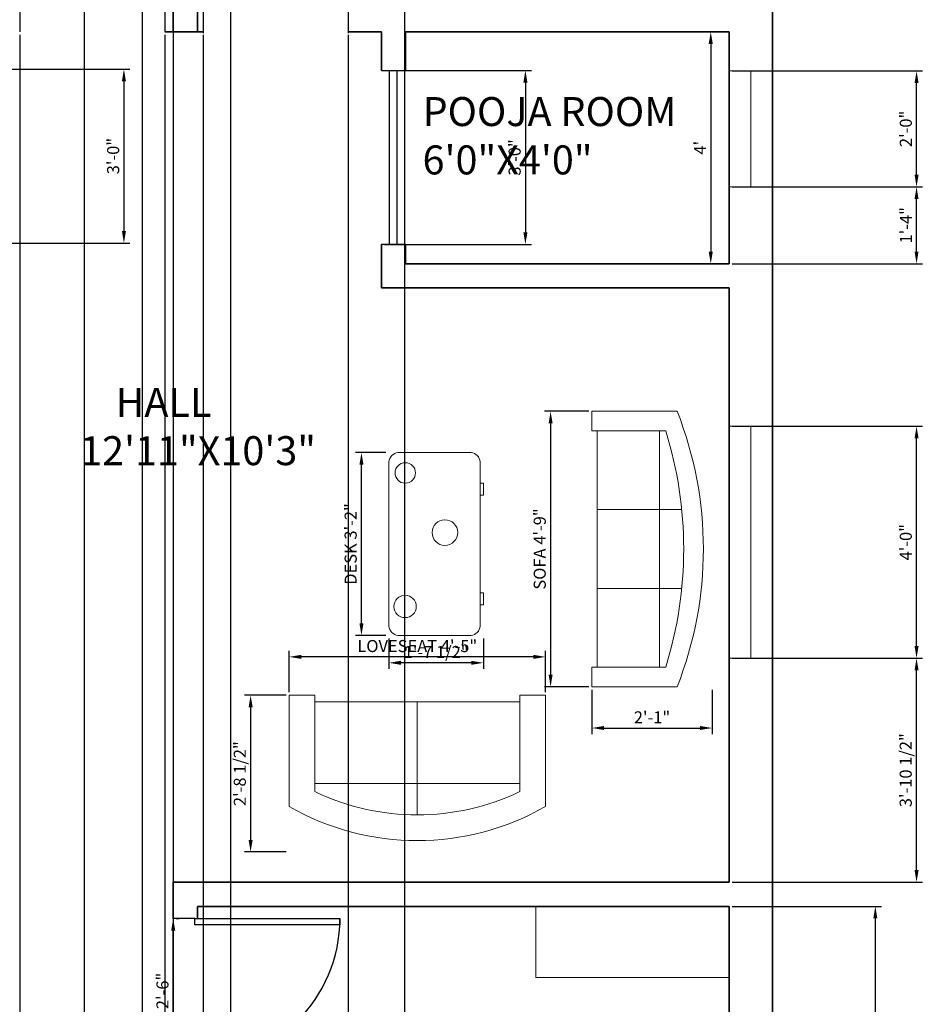
# Model space of a CAD drawing. Units: inches. Extents: x 3889 to 4254, y 3310 to 3958.
# Tile 4 of 6: x 4067 to 4254, y 3534 to 3738. Entities that reach past the tile are written whole.
import ezdxf

# ---------------------------------------------------------------- set-up
doc = ezdxf.new("R2010")
doc.units = ezdxf.units.IN
for name, color, linetype, lineweight in [('A-AREA-IDEN', 11, 'Continuous', 18), ('A-WALL', 7, 'Continuous', 35), ('DIM', 81, 'Continuous', 18), ('DOOR', 1, 'Continuous', 25), ('FURNITURES', 130, 'Continuous', 18), ('WINDOW', 3, 'Continuous', 18)]:
    doc.layers.add(name, color=color, linetype=linetype, lineweight=lineweight)
doc.styles.get("Standard").update_dxf_attribs({"font": 'arial.ttf'})
doc.dimstyles.new('ISO-25', dxfattribs={"dimtxt": 2.5, "dimasz": 2.5, "dimexe": 1.25, "dimexo": 0.625, "dimtad": 1, "dimlunit": 3, "dimtxsty": 'Standard', "dimcen": 2.5, "dimadec": 0, "dimazin": 0, "dimtfac": 1, "dimtmove": 0, "dimatfit": 3, "dimfxl": 1, "dimarcsym": 0})

# ---------------------------------------------------------------- blocks, each defined once
blk = doc.blocks.new('*U4')
for p, q in [((0, 0), (0, -6)), ((40, 0), (40, -6))]:
    blk.add_line(p, q)
blk.add_lwpolyline([(0, 0), (0, 40), (1.75, 40), (1.75, 0)], close=True)
blk.add_arc((0, 0), 40, 0, 90)
blk = doc.blocks.new('*U2')
for p, q in [((0, 0), (0, -6)), ((-40, 0), (-40, -6))]:
    blk.add_line(p, q)
blk.add_lwpolyline([(0, 0), (0, 40), (-1.75, 40), (-1.75, 0)], close=True)
blk.add_arc((0, 0), 40, 90, 180)
blk = doc.blocks.new('*U3')
for p, q in [((-40, 0), (-40, 6)), ((0, 0), (0, 6))]:
    blk.add_line(p, q)
blk.add_lwpolyline([(0, 0), (0, -40), (-1.75, -40), (-1.75, 0)], close=True)
blk.add_arc((0, 0), 40, 180, 270)
blk = doc.blocks.new('Desk - 30 x 60 in.')
for p, q in [((-26.999995, 0), (26.999995, 0)), ((-29.999995, -27), (-29.999995, -3)), ((29.999995, -3), (29.999995, -27)), ((26.999995, -30), (-26.999995, -30)), ((-20.000005, -30), (-20.000005, -31)), ((-20.000005, -31), (-16.000005, -31)), ((-16.000005, -31), (-16.000005, -30)), ((15.999995, -31), (15.999995, -30)), ((19.999995, -31), (15.999995, -31)), ((19.999995, -30), (19.999995, -31))]:
    blk.add_line(p, q)
for centre, start, end in [((-26.499995, -3.5), 98.1301, 171.8699), ((26.499995, -3.5), 8.130102, 81.8699), ((-26.499995, -26.5), 188.1301, 261.8699), ((26.499995, -26.5), 278.1301, 351.8699)]:
    blk.add_arc(centre, 3.535534, start, end)
blk = doc.blocks.new('Sofa - Roundback 7 ft.')
for p, q in [((-12.00002, -32.4421), (-12.00003, -6.5971)), ((11.99997, -32.4421), (11.99998, -6.5971)), ((-36.000027, -34), (-36.000027, -11.4696)), ((35.99998, -34), (35.99998, -11.4696)), ((-35.999844, -13.3819), (35.9998, -13.3819)), ((-36.000027, -32.4421), (35.99998, -32.4421))]:
    blk.add_line(p, q)
for points in [[(-36.000027, -34), (-42.000027, -34), (-42.000027, -8)], [(41.99998, -8), (41.99998, -34), (35.99998, -34)]]:
    blk.add_lwpolyline(points)
for centre, radius, start, end in [((0, -114.25), 114.25, 68.43141, 111.5686), ((-0.00001, -127.1968), 121.1968, 72.72033, 107.2797)]:
    blk.add_arc(centre, radius, start, end)
blk = doc.blocks.new('Sofa - Roundback Loveseat 5 ft.')
for p, q in [((0, -32.44198), (0, -5.99998)), ((-24, -33.99998), (-24, -11.46958)), ((24.00004, -33.99998), (24.00004, -11.46958)), ((-23.9998, -13.38178), (23.99986, -13.38178)), ((-24, -32.44198), (24.00004, -32.44198))]:
    blk.add_line(p, q)
for points in [[(-24, -33.99998), (-30, -33.99998), (-30, -7.99998)], [(30.00004, -7.99998), (30.00004, -33.99998), (24.00004, -33.99998)]]:
    blk.add_lwpolyline(points)
for centre, radius, start, end in [((0, -60.24998), 60.24998, 60.13715, 119.8628), ((0, -61.38438), 55.38444, 64.32083, 115.6792)]:
    blk.add_arc(centre, radius, start, end)
blk = doc.blocks.new('*D27')
at = {"layer": 'Defpoints', "color": 0, "transparency": 16777216}
for p in [(4098.84, 3551.61), (4098.84, 3551.61), (4098.84, 3521.61)]:
    blk.add_point(p, dxfattribs=at)
at = {"layer": 'DIM', "color": 0, "lineweight": -2, "transparency": 16777216}
for p, q in [((4099.47, 3551.61), (4100.09, 3551.61)), ((4098.84, 3524.11), (4098.84, 3549.11)), ((4099.47, 3521.61), (4100.09, 3521.61))]:
    blk.add_line(p, q, dxfattribs=at)
at = {"layer": 'DIM', "color": 0, "transparency": 16777216}
for points in [[(4098.43, 3549.11), (4099.26, 3549.11), (4098.84, 3551.61)], [(4098.43, 3524.11), (4099.26, 3524.11), (4098.84, 3521.61)]]:
    blk.add_solid(points, dxfattribs=at)
at = {"layer": 'DIM', "color": 0, "transparency": 16777216, "insert": (4096.94, 3536.61), "char_height": 2.5, "attachment_point": 5, "rotation": 90}
blk.add_mtext('2\'-6"', dxfattribs=at)
blk = doc.blocks.new('*D29')
at = {"layer": 'Defpoints', "color": 0, "transparency": 16777216}
for p in [(4213.84, 3554.11), (4213.84, 3434.11), (4244.11, 3434.11)]:
    blk.add_point(p, dxfattribs=at)
at = {"layer": 'DIM', "color": 0, "lineweight": -2, "transparency": 16777216}
for p, q in [((4214.47, 3554.11), (4245.36, 3554.11)), ((4244.11, 3551.61), (4244.11, 3436.61)), ((4214.47, 3434.11), (4245.36, 3434.11))]:
    blk.add_line(p, q, dxfattribs=at)
at = {"layer": 'DIM', "color": 0, "transparency": 16777216}
for points in [[(4243.7, 3551.61), (4244.53, 3551.61), (4244.11, 3554.11)], [(4243.7, 3436.61), (4244.53, 3436.61), (4244.11, 3434.11)]]:
    blk.add_solid(points, dxfattribs=at)
at = {"layer": 'DIM', "color": 0, "transparency": 16777216, "insert": (4242.21, 3494.11), "char_height": 2.5, "attachment_point": 5, "rotation": 90}
blk.add_mtext("10'", dxfattribs=at)
blk = doc.blocks.new('*D30')
at = {"layer": 'Defpoints', "color": 0, "transparency": 16777216}
for p in [(4208.35, 3735.11), (4208.35, 3687.11), (4210.06, 3687.11)]:
    blk.add_point(p, dxfattribs=at)
at = {"layer": 'DIM', "color": 0, "lineweight": -2, "transparency": 16777216}
for p, q in [((4208.98, 3735.11), (4211.31, 3735.11)), ((4210.06, 3732.61), (4210.06, 3689.61)), ((4208.98, 3687.11), (4211.31, 3687.11))]:
    blk.add_line(p, q, dxfattribs=at)
at = {"layer": 'DIM', "color": 0, "transparency": 16777216}
for points in [[(4209.64, 3732.61), (4210.48, 3732.61), (4210.06, 3735.11)], [(4209.64, 3689.61), (4210.48, 3689.61), (4210.06, 3687.11)]]:
    blk.add_solid(points, dxfattribs=at)
at = {"layer": 'DIM', "color": 0, "transparency": 16777216, "insert": (4208.18, 3711.11), "char_height": 2.5, "attachment_point": 5, "rotation": 90}
blk.add_mtext("4'", dxfattribs=at)
blk = doc.blocks.new('WIN-48x9')
blk.add_line((4.5, 48), (4.5, 0))
blk.add_lwpolyline([(0, 48), (9, 48), (9, 0), (0, 0)], close=True)
blk = doc.blocks.new('WIN-24x9')
blk.add_line((24, 4.5), (0, 4.5))
blk.add_lwpolyline([(24, 9), (24, 0), (0, 0), (0, 9)], close=True)
blk = doc.blocks.new('*D53')
at = {"layer": 'Defpoints', "color": 0, "transparency": 16777216}
for p in [(4137.79, 3648.02), (4143.47, 3648.02), (4143.47, 3610.19)]:
    blk.add_point(p, dxfattribs=at)
at = {"layer": 'DIM', "color": 0, "lineweight": -2, "transparency": 16777216}
for p, q in [((4142.84, 3648.02), (4136.54, 3648.02)), ((4137.79, 3612.69), (4137.79, 3645.52)), ((4142.84, 3610.19), (4136.54, 3610.19))]:
    blk.add_line(p, q, dxfattribs=at)
at = {"layer": 'DIM', "color": 0, "transparency": 16777216}
for points in [[(4137.38, 3645.52), (4138.21, 3645.52), (4137.79, 3648.02)], [(4137.38, 3612.69), (4138.21, 3612.69), (4137.79, 3610.19)]]:
    blk.add_solid(points, dxfattribs=at)
at = {"layer": 'DIM', "color": 0, "transparency": 16777216, "insert": (4135.88, 3629.1), "char_height": 2.5, "attachment_point": 5, "rotation": 90}
blk.add_mtext('DESK 3\'-2"', dxfattribs=at)
blk = doc.blocks.new('*D54')
at = {"layer": 'Defpoints', "color": 0, "transparency": 16777216}
for p in [(4143.47, 3610.19), (4163.01, 3610.19), (4143.47, 3604.51)]:
    blk.add_point(p, dxfattribs=at)
at = {"layer": 'DIM', "color": 0, "lineweight": -2, "transparency": 16777216}
for p, q in [((4143.47, 3609.56), (4143.47, 3603.26)), ((4163.01, 3609.56), (4163.01, 3603.26)), ((4160.51, 3604.51), (4145.97, 3604.51))]:
    blk.add_line(p, q, dxfattribs=at)
at = {"layer": 'DIM', "color": 0, "transparency": 16777216}
for points in [[(4145.97, 3604.93), (4145.97, 3604.1), (4143.47, 3604.51)], [(4160.51, 3604.93), (4160.51, 3604.1), (4163.01, 3604.51)]]:
    blk.add_solid(points, dxfattribs=at)
at = {"layer": 'DIM', "color": 0, "transparency": 16777216, "insert": (4153.24, 3606.43), "char_height": 2.5, "attachment_point": 5}
blk.add_mtext('1\'-7 1/2"', dxfattribs=at)
blk = doc.blocks.new('*D55')
at = {"layer": 'Defpoints', "color": 0, "transparency": 16777216}
for p in [(4185.47, 3656.56), (4176.92, 3599.57), (4185.47, 3599.57)]:
    blk.add_point(p, dxfattribs=at)
at = {"layer": 'DIM', "color": 0, "lineweight": -2, "transparency": 16777216}
for p, q in [((4184.85, 3656.56), (4175.67, 3656.56)), ((4176.92, 3654.06), (4176.92, 3602.07)), ((4184.85, 3599.57), (4175.67, 3599.57))]:
    blk.add_line(p, q, dxfattribs=at)
at = {"layer": 'DIM', "color": 0, "transparency": 16777216}
for points in [[(4176.51, 3654.06), (4177.34, 3654.06), (4176.92, 3656.56)], [(4176.51, 3602.07), (4177.34, 3602.07), (4176.92, 3599.57)]]:
    blk.add_solid(points, dxfattribs=at)
at = {"layer": 'DIM', "color": 0, "transparency": 16777216, "insert": (4175, 3628.07), "char_height": 2.5, "attachment_point": 5, "rotation": 90}
blk.add_mtext('SOFA 4\'-9"', dxfattribs=at)
blk = doc.blocks.new('*D56')
at = {"layer": 'Defpoints', "color": 0, "transparency": 16777216}
for p in [(4185.47, 3599.57), (4210.35, 3599.57), (4210.35, 3591.02)]:
    blk.add_point(p, dxfattribs=at)
at = {"layer": 'DIM', "color": 0, "lineweight": -2, "transparency": 16777216}
for p, q in [((4185.47, 3598.95), (4185.47, 3589.77)), ((4210.35, 3598.95), (4210.35, 3589.77)), ((4187.97, 3591.02), (4207.85, 3591.02))]:
    blk.add_line(p, q, dxfattribs=at)
at = {"layer": 'DIM', "color": 0, "transparency": 16777216}
for points in [[(4187.97, 3591.44), (4187.97, 3590.61), (4185.47, 3591.02)], [(4207.85, 3591.44), (4207.85, 3590.61), (4210.35, 3591.02)]]:
    blk.add_solid(points, dxfattribs=at)
at = {"layer": 'DIM', "color": 0, "transparency": 16777216, "insert": (4197.91, 3592.9), "char_height": 2.5, "attachment_point": 5}
blk.add_mtext('2\'-1"', dxfattribs=at)
blk = doc.blocks.new('*D57')
at = {"layer": 'Defpoints', "color": 0, "transparency": 16777216}
for p in [(4122.82, 3605.74), (4122.82, 3597.79), (4175.87, 3597.79)]:
    blk.add_point(p, dxfattribs=at)
at = {"layer": 'DIM', "color": 0, "lineweight": -2, "transparency": 16777216}
for p, q in [((4122.82, 3598.41), (4122.82, 3606.99)), ((4175.87, 3598.41), (4175.87, 3606.99)), ((4173.37, 3605.74), (4125.32, 3605.74))]:
    blk.add_line(p, q, dxfattribs=at)
at = {"layer": 'DIM', "color": 0, "transparency": 16777216}
for points in [[(4125.32, 3606.16), (4125.32, 3605.33), (4122.82, 3605.74)], [(4173.37, 3606.16), (4173.37, 3605.33), (4175.87, 3605.74)]]:
    blk.add_solid(points, dxfattribs=at)
at = {"layer": 'DIM', "color": 0, "transparency": 16777216, "insert": (4149.34, 3607.66), "char_height": 2.5, "attachment_point": 5}
blk.add_mtext('LOVESEAT 4\'-5"', dxfattribs=at)
blk = doc.blocks.new('*D58')
at = {"layer": 'Defpoints', "color": 0, "transparency": 16777216}
for p in [(4122.82, 3597.79), (4114.86, 3565.37), (4122.82, 3565.37)]:
    blk.add_point(p, dxfattribs=at)
at = {"layer": 'DIM', "color": 0, "lineweight": -2, "transparency": 16777216}
for p, q in [((4122.19, 3597.79), (4113.61, 3597.79)), ((4114.86, 3595.29), (4114.86, 3567.87)), ((4122.19, 3565.37), (4113.61, 3565.37))]:
    blk.add_line(p, q, dxfattribs=at)
at = {"layer": 'DIM', "color": 0, "transparency": 16777216}
for points in [[(4114.44, 3595.29), (4115.28, 3595.29), (4114.86, 3597.79)], [(4114.44, 3567.87), (4115.28, 3567.87), (4114.86, 3565.37)]]:
    blk.add_solid(points, dxfattribs=at)
at = {"layer": 'DIM', "color": 0, "transparency": 16777216, "insert": (4112.94, 3581.58), "char_height": 2.5, "attachment_point": 5, "rotation": 90}
blk.add_mtext('2\'-8 1/2"', dxfattribs=at)
blk = doc.blocks.new('*D71')
at = {"layer": 'Defpoints', "color": 0, "transparency": 16777216}
for p in [(4092.52, 3951.91), (4080.52, 3351.11), (4092.52, 3351.11)]:
    blk.add_point(p, dxfattribs=at)
at = {"layer": 'DIM', "color": 0, "lineweight": -2, "transparency": 16777216}
for p, q in [((4080.52, 3351.73), (4080.52, 3953.16)), ((4092.52, 3351.73), (4092.52, 3953.16)), ((4083.02, 3951.91), (4090.02, 3951.91))]:
    blk.add_line(p, q, dxfattribs=at)
at = {"layer": 'DIM', "color": 0, "transparency": 16777216}
for points in [[(4083.02, 3952.32), (4083.02, 3951.49), (4080.52, 3951.91)], [(4090.02, 3952.32), (4090.02, 3951.49), (4092.52, 3951.91)]]:
    blk.add_solid(points, dxfattribs=at)
at = {"layer": 'DIM', "color": 0, "transparency": 16777216, "insert": (4086.52, 3953.81), "char_height": 2.5, "attachment_point": 5}
blk.add_mtext('1\'-0"', dxfattribs=at)
blk = doc.blocks.new('*D78')
at = {"layer": 'Defpoints', "color": 0, "transparency": 16777216}
for p in [(4213.84, 3703.01), (4252.64, 3703.01), (4213.84, 3687.11)]:
    blk.add_point(p, dxfattribs=at)
at = {"layer": 'DIM', "color": 0, "lineweight": -2, "transparency": 16777216}
for p, q in [((4214.47, 3703.01), (4253.89, 3703.01)), ((4252.64, 3689.61), (4252.64, 3700.51)), ((4214.47, 3687.11), (4253.89, 3687.11))]:
    blk.add_line(p, q, dxfattribs=at)
at = {"layer": 'DIM', "color": 0, "transparency": 16777216}
for points in [[(4252.23, 3700.51), (4253.06, 3700.51), (4252.64, 3703.01)], [(4252.23, 3689.61), (4253.06, 3689.61), (4252.64, 3687.11)]]:
    blk.add_solid(points, dxfattribs=at)
at = {"layer": 'DIM', "color": 0, "transparency": 16777216, "insert": (4250.76, 3695.06), "char_height": 2.5, "attachment_point": 5, "rotation": 90}
blk.add_mtext('1\'-4"', dxfattribs=at)
blk = doc.blocks.new('*D79')
at = {"layer": 'Defpoints', "color": 0, "transparency": 16777216}
for p in [(4213.84, 3605.47), (4252.64, 3605.47), (4213.84, 3559.11)]:
    blk.add_point(p, dxfattribs=at)
at = {"layer": 'DIM', "color": 0, "lineweight": -2, "transparency": 16777216}
for p, q in [((4214.47, 3605.47), (4253.89, 3605.47)), ((4252.64, 3561.61), (4252.64, 3602.97)), ((4214.47, 3559.11), (4253.89, 3559.11))]:
    blk.add_line(p, q, dxfattribs=at)
at = {"layer": 'DIM', "color": 0, "transparency": 16777216}
for points in [[(4252.23, 3602.97), (4253.06, 3602.97), (4252.64, 3605.47)], [(4252.23, 3561.61), (4253.06, 3561.61), (4252.64, 3559.11)]]:
    blk.add_solid(points, dxfattribs=at)
at = {"layer": 'DIM', "color": 0, "transparency": 16777216, "insert": (4250.72, 3582.29), "char_height": 2.5, "attachment_point": 5, "rotation": 90}
blk.add_mtext('3\'-10 1/2"', dxfattribs=at)
blk = doc.blocks.new('*D83')
at = {"layer": 'Defpoints', "color": 0, "transparency": 16777216}
for p in [(4213.84, 3653.47), (4252.64, 3653.47), (4213.84, 3605.47)]:
    blk.add_point(p, dxfattribs=at)
at = {"layer": 'DIM', "color": 0, "lineweight": -2, "transparency": 16777216}
for p, q in [((4214.47, 3653.47), (4253.89, 3653.47)), ((4252.64, 3607.97), (4252.64, 3650.97)), ((4214.47, 3605.47), (4253.89, 3605.47))]:
    blk.add_line(p, q, dxfattribs=at)
at = {"layer": 'DIM', "color": 0, "transparency": 16777216}
for points in [[(4252.23, 3650.97), (4253.06, 3650.97), (4252.64, 3653.47)], [(4252.23, 3607.97), (4253.06, 3607.97), (4252.64, 3605.47)]]:
    blk.add_solid(points, dxfattribs=at)
at = {"layer": 'DIM', "color": 0, "transparency": 16777216, "insert": (4250.74, 3629.47), "char_height": 2.5, "attachment_point": 5, "rotation": 90}
blk.add_mtext('4\'-0"', dxfattribs=at)
blk = doc.blocks.new('*D84')
at = {"layer": 'Defpoints', "color": 0, "transparency": 16777216}
for p in [(4213.84, 3727.01), (4252.64, 3727.01), (4213.84, 3703.01)]:
    blk.add_point(p, dxfattribs=at)
at = {"layer": 'DIM', "color": 0, "lineweight": -2, "transparency": 16777216}
for p, q in [((4214.47, 3727.01), (4253.89, 3727.01)), ((4252.64, 3705.51), (4252.64, 3724.51)), ((4214.47, 3703.01), (4253.89, 3703.01))]:
    blk.add_line(p, q, dxfattribs=at)
at = {"layer": 'DIM', "color": 0, "transparency": 16777216}
for points in [[(4252.23, 3724.51), (4253.06, 3724.51), (4252.64, 3727.01)], [(4252.23, 3705.51), (4253.06, 3705.51), (4252.64, 3703.01)]]:
    blk.add_solid(points, dxfattribs=at)
at = {"layer": 'DIM', "color": 0, "transparency": 16777216, "insert": (4250.74, 3715.01), "char_height": 2.5, "attachment_point": 5, "rotation": 90}
blk.add_mtext('2\'-0"', dxfattribs=at)
blk = doc.blocks.new('*D85')
at = {"layer": 'Defpoints', "color": 0, "transparency": 16777216}
for p in [(4110.69, 3860.11), (4146.69, 3860.11), (4146.69, 3312.31)]:
    blk.add_point(p, dxfattribs=at)
at = {"layer": 'DIM', "color": 0, "lineweight": -2, "transparency": 16777216}
for p, q in [((4110.69, 3859.48), (4110.69, 3311.06)), ((4146.69, 3859.48), (4146.69, 3311.06)), ((4113.19, 3312.31), (4144.19, 3312.31))]:
    blk.add_line(p, q, dxfattribs=at)
at = {"layer": 'DIM', "color": 0, "transparency": 16777216}
for points in [[(4113.19, 3312.72), (4113.19, 3311.89), (4110.69, 3312.31)], [(4144.19, 3312.72), (4144.19, 3311.89), (4146.69, 3312.31)]]:
    blk.add_solid(points, dxfattribs=at)
at = {"layer": 'DIM', "color": 0, "transparency": 16777216, "insert": (4128.69, 3314.21), "char_height": 2.5, "attachment_point": 5}
blk.add_mtext('3\'-0"', dxfattribs=at)
blk = doc.blocks.new('*D86')
at = {"layer": 'Defpoints', "color": 0, "transparency": 16777216}
for p in [(4046.84, 3865.11), (4110.69, 3865.11), (4110.69, 3312.31)]:
    blk.add_point(p, dxfattribs=at)
at = {"layer": 'DIM', "color": 0, "lineweight": -2, "transparency": 16777216}
for p, q in [((4046.84, 3864.48), (4046.84, 3311.06)), ((4110.69, 3864.48), (4110.69, 3311.06)), ((4049.34, 3312.31), (4108.19, 3312.31))]:
    blk.add_line(p, q, dxfattribs=at)
at = {"layer": 'DIM', "color": 0, "transparency": 16777216}
for points in [[(4049.34, 3312.72), (4049.34, 3311.89), (4046.84, 3312.31)], [(4108.19, 3312.72), (4108.19, 3311.89), (4110.69, 3312.31)]]:
    blk.add_solid(points, dxfattribs=at)
at = {"layer": 'DIM', "color": 0, "transparency": 16777216, "insert": (4078.77, 3314.2), "char_height": 2.5, "attachment_point": 5}
blk.add_mtext('5\'-4"', dxfattribs=at)
blk = doc.blocks.new('*D87')
at = {"layer": 'Defpoints', "color": 0, "transparency": 16777216}
for p in [(4058.84, 3727.38), (4058.84, 3691.38), (4088.64, 3691.38)]:
    blk.add_point(p, dxfattribs=at)
at = {"layer": 'DIM', "color": 0, "lineweight": -2, "transparency": 16777216}
for p, q in [((4059.47, 3727.38), (4089.89, 3727.38)), ((4088.64, 3724.88), (4088.64, 3693.88)), ((4059.47, 3691.38), (4089.89, 3691.38))]:
    blk.add_line(p, q, dxfattribs=at)
at = {"layer": 'DIM', "color": 0, "transparency": 16777216}
for points in [[(4088.23, 3724.88), (4089.06, 3724.88), (4088.64, 3727.38)], [(4088.23, 3693.88), (4089.06, 3693.88), (4088.64, 3691.38)]]:
    blk.add_solid(points, dxfattribs=at)
at = {"layer": 'DIM', "color": 0, "transparency": 16777216, "insert": (4086.74, 3709.38), "char_height": 2.5, "attachment_point": 5, "rotation": 90}
blk.add_mtext('3\'-0"', dxfattribs=at)
blk = doc.blocks.new('*D88')
at = {"layer": 'Defpoints', "color": 0, "transparency": 16777216}
for p in [(4141.91, 3727.1), (4141.91, 3691.1), (4171.71, 3691.1)]:
    blk.add_point(p, dxfattribs=at)
at = {"layer": 'DIM', "color": 0, "lineweight": -2, "transparency": 16777216}
for p, q in [((4142.53, 3727.1), (4172.96, 3727.1)), ((4171.71, 3724.6), (4171.71, 3693.6)), ((4142.53, 3691.1), (4172.96, 3691.1))]:
    blk.add_line(p, q, dxfattribs=at)
at = {"layer": 'DIM', "color": 0, "transparency": 16777216}
for points in [[(4171.29, 3724.6), (4172.13, 3724.6), (4171.71, 3727.1)], [(4171.29, 3693.6), (4172.13, 3693.6), (4171.71, 3691.1)]]:
    blk.add_solid(points, dxfattribs=at)
at = {"layer": 'DIM', "color": 0, "transparency": 16777216, "insert": (4169.81, 3709.1), "char_height": 2.5, "attachment_point": 5, "rotation": 90}
blk.add_mtext('3\'-0"', dxfattribs=at)
blk = doc.blocks.new('*D89')
at = {"layer": 'Defpoints', "color": 0, "transparency": 16777216}
for p in [(4067.08, 3735.11), (4097.08, 3735.11), (4097.08, 3312.31)]:
    blk.add_point(p, dxfattribs=at)
at = {"layer": 'DIM', "color": 0, "lineweight": -2, "transparency": 16777216}
for p, q in [((4067.08, 3734.48), (4067.08, 3311.06)), ((4097.08, 3734.48), (4097.08, 3311.06)), ((4069.58, 3312.31), (4094.58, 3312.31))]:
    blk.add_line(p, q, dxfattribs=at)
at = {"layer": 'DIM', "color": 0, "transparency": 16777216}
for points in [[(4069.58, 3312.72), (4069.58, 3311.89), (4067.08, 3312.31)], [(4094.58, 3312.72), (4094.58, 3311.89), (4097.08, 3312.31)]]:
    blk.add_solid(points, dxfattribs=at)
at = {"layer": 'DIM', "color": 0, "transparency": 16777216, "insert": (4082.08, 3314.21), "char_height": 2.5, "attachment_point": 5}
blk.add_mtext('2\'-6"', dxfattribs=at)
blk = doc.blocks.new('*D90')
at = {"layer": 'Defpoints', "color": 0, "transparency": 16777216}
for p in [(4105.04, 3735.11), (4135.04, 3735.11), (4135.04, 3312.31)]:
    blk.add_point(p, dxfattribs=at)
at = {"layer": 'DIM', "color": 0, "lineweight": -2, "transparency": 16777216}
for p, q in [((4105.04, 3734.48), (4105.04, 3311.06)), ((4135.04, 3734.48), (4135.04, 3311.06)), ((4107.54, 3312.31), (4132.54, 3312.31))]:
    blk.add_line(p, q, dxfattribs=at)
at = {"layer": 'DIM', "color": 0, "transparency": 16777216}
for points in [[(4107.54, 3312.72), (4107.54, 3311.89), (4105.04, 3312.31)], [(4132.54, 3312.72), (4132.54, 3311.89), (4135.04, 3312.31)]]:
    blk.add_solid(points, dxfattribs=at)
at = {"layer": 'DIM', "color": 0, "transparency": 16777216, "insert": (4120.04, 3314.21), "char_height": 2.5, "attachment_point": 5}
blk.add_mtext('2\'-6"', dxfattribs=at)
blk = doc.blocks.new('*D95')
at = {"layer": 'Defpoints', "color": 0, "transparency": 16777216}
for p in [(4046.84, 3865.11), (4098.84, 3860.11), (4098.84, 3312.31)]:
    blk.add_point(p, dxfattribs=at)
at = {"layer": 'DIM', "color": 0, "lineweight": -2, "transparency": 16777216}
for p, q in [((4046.84, 3864.48), (4046.84, 3311.06)), ((4098.84, 3859.48), (4098.84, 3311.06)), ((4049.34, 3312.31), (4096.34, 3312.31))]:
    blk.add_line(p, q, dxfattribs=at)
at = {"layer": 'DIM', "color": 0, "transparency": 16777216}
for points in [[(4049.34, 3312.72), (4049.34, 3311.89), (4046.84, 3312.31)], [(4096.34, 3312.72), (4096.34, 3311.89), (4098.84, 3312.31)]]:
    blk.add_solid(points, dxfattribs=at)
at = {"layer": 'DIM', "color": 0, "transparency": 16777216, "insert": (4072.84, 3314.18), "char_height": 2.5, "attachment_point": 5}
blk.add_mtext('4\'-4"', dxfattribs=at)

msp = doc.modelspace()

# ---------------------------------------------------------------- linework, layer by layer
at = {"layer": 'A-WALL'}
for p, q in [((4222.843, 3342.107), (4222.843, 3922.107)), ((4098.843, 3735.107), (4098.843, 3860.107)), ((4103.843, 3735.107), (4103.843, 3860.107)), ((4097.08, 3735.107), (4103.843, 3735.107)), ((4098.843, 3735.107), (4103.843, 3735.107)), ((4103.843, 3735.107), (4105.044, 3735.107)), ((4135.044, 3735.107), (4141.91, 3735.107)), ((4141.91, 3727.102), (4141.91, 3735.107)), ((4146.91, 3727.102), (4146.91, 3735.107)), ((4146.91, 3735.107), (4213.843, 3735.107)), ((4213.843, 3687.107), (4213.843, 3735.107)), ((4141.91, 3682.107), (4141.91, 3691.102)), ((4146.91, 3687.107), (4146.91, 3691.102)), ((4146.91, 3687.107), (4213.843, 3687.107)), ((4141.91, 3682.107), (4213.843, 3682.107)), ((4213.843, 3559.107), (4213.843, 3682.107)), ((4098.843, 3559.107), (4213.843, 3559.107)), ((4098.843, 3551.612), (4098.843, 3559.107)), ((4103.843, 3554.107), (4213.843, 3554.107)), ((4103.843, 3551.612), (4103.843, 3554.107)), ((4213.843, 3434.107), (4213.843, 3554.107))]:
    msp.add_line(p, q, dxfattribs=at)
at = {"layer": 'DOOR'}
for points in [[(4141.91, 3727.102), (4146.91, 3727.102)], [(4146.91, 3691.102), (4141.91, 3691.102)]]:
    msp.add_lwpolyline(points, dxfattribs=at)
msp.add_lwpolyline([(4143.572, 3727.102), (4145.076, 3727.102), (4145.076, 3691.102), (4143.572, 3691.102)], close=True, dxfattribs=at)
at = {"layer": 'FURNITURES'}
msp.add_lwpolyline([(4213.843, 3554.107), (4173.893, 3554.107), (4173.893, 3539.394), (4213.843, 3539.394)], close=True, dxfattribs=at)
for centre, radius in [((4146.861, 3643.814), 2.119), ((4155.058, 3631.466), 2.655), ((4146.809, 3616.181), 2.318)]:
    msp.add_circle(centre, radius, dxfattribs=at)

# ---------------------------------------------------------------- block references
at = {"layer": 'DOOR', "xscale": 0.75, "yscale": 0.75, "zscale": 0.75}
for name, p in [('*U2', (4097.08, 3739.607)), ('*U4', (4105.044, 3739.339))]:
    msp.add_blockref(name, p, dxfattribs=at)
at = {"layer": 'DOOR', "xscale": 0.75, "yscale": 0.75, "zscale": 0.75, "rotation": 90}
msp.add_blockref('*U3', (4103.343, 3551.612), dxfattribs=at)
at = {"layer": 'FURNITURES'}
for name, p, xscale, yscale, zscale, rotation in [('Sofa - Roundback 7 ft.', (4208.538, 3628.068), 0.6784518660872728, 0.6784518660872728, 0.6784518660872728, 270), ('Desk - 30 x 60 in.', (4143.468, 3629.103), 0.6305181038195912, 0.6305181038195912, 0.6305181038195912, 90), ('Sofa - Roundback Loveseat 5 ft.', (4149.343, 3567.724), 0.8841712959600512, 0.8841712959600512, 0.8841712959600512, 180)]:
    msp.add_blockref(name, p, dxfattribs=dict(at, xscale=xscale, yscale=yscale, zscale=zscale, rotation=rotation))
at = {"layer": 'WINDOW', "rotation": 89.99999999999939}
msp.add_blockref('WIN-24x9', (4222.843, 3703.007), dxfattribs=at)
at = {"layer": 'WINDOW'}
msp.add_blockref('WIN-48x9', (4213.843, 3605.469), dxfattribs=at)

# ---------------------------------------------------------------- texts
at = {"layer": 'A-AREA-IDEN', "char_height": 6, "attachment_point": 1}
for s, insert in [('POOJA ROOM\\P6\'0"X4\'0"', (4150.436, 3721.593)), ('    HALL\\P12\'11"X10\'3"', (4079.585, 3661.416))]:
    msp.add_mtext_dynamic_manual_height_columns(s, width=76.4548, gutter_width=12.5, heights=[0], dxfattribs=dict(at, insert=insert))

# ---------------------------------------------------------------- dimensions: what is measured, and where the dimension line sits
at = {"layer": 'DIM'}
for base, p1, p2, picture, middle in [((4092.518, 3951.907), (4080.518, 3351.107), (4092.518, 3351.107), '*D71', (4086.518, 3953.808)), ((4110.69, 3312.307), (4046.843, 3865.107), (4110.69, 3865.107), '*D86', (4078.766, 3314.203)), ((4098.843, 3312.307), (4046.843, 3865.107), (4098.843, 3860.107), '*D95', (4072.843, 3314.182)), ((4146.69, 3312.307), (4110.69, 3860.107), (4146.69, 3860.107), '*D85', (4128.69, 3314.209)), ((4097.08, 3312.307), (4067.08, 3735.107), (4097.08, 3735.107), '*D89', (4082.08, 3314.208)), ((4135.044, 3312.307), (4105.044, 3735.107), (4135.044, 3735.107), '*D90', (4120.044, 3314.208)), ((4210.348, 3591.025), (4185.471, 3599.573), (4210.348, 3599.573), '*D56', (4197.909, 3592.905))]:
    dim = msp.add_linear_dim(base=base, p1=p1, p2=p2, dimstyle='ISO-25', override={"dimdec": 1, "dimlfac": 1, "dimrnd": 0, "dimzin": 1, "dimdsep": 46, "dimlunit": 4, "dimfrac": 2}, dxfattribs=at)
    dim.commit()
    dim.dimension.update_dxf_attribs({"geometry": picture, "text_midpoint": middle})
for base, p1, p2, angle, override, picture, middle in [((4210.06, 3687.107), (4208.353, 3735.107), (4208.353, 3687.107), 90, {"dimclrd": 0, "dimclre": 0, "dimclrt": 0}, '*D30', (4208.185, 3711.107)), ((4088.643, 3691.381), (4058.843, 3727.381), (4058.843, 3691.381), 270, {"dimdec": 1, "dimlfac": 1, "dimrnd": 0, "dimzin": 1, "dimdsep": 46, "dimlunit": 4, "dimfrac": 2}, '*D87', (4086.741, 3709.381)), ((4171.71, 3691.102), (4141.91, 3727.102), (4141.91, 3691.102), 270, {"dimdec": 1, "dimlfac": 1, "dimrnd": 0, "dimzin": 1, "dimdsep": 46, "dimlunit": 4, "dimfrac": 2}, '*D88', (4169.807, 3709.102)), ((4252.643, 3727.007), (4213.843, 3703.007), (4213.843, 3727.007), 90, {"dimdec": 1, "dimlfac": 1, "dimrnd": 0, "dimzin": 1, "dimdsep": 46, "dimlunit": 4, "dimfrac": 2}, '*D84', (4250.741, 3715.007)), ((4252.643, 3703.007), (4213.843, 3687.107), (4213.843, 3703.007), 90, {"dimdec": 1, "dimlfac": 1, "dimrnd": 0, "dimzin": 1, "dimdsep": 46, "dimlunit": 4, "dimfrac": 2}, '*D78', (4250.763, 3695.057)), ((4252.643, 3653.469), (4213.843, 3605.469), (4213.843, 3653.469), 90, {"dimdec": 1, "dimlfac": 1, "dimrnd": 0, "dimzin": 1, "dimdsep": 46, "dimlunit": 4, "dimfrac": 2}, '*D83', (4250.741, 3629.469)), ((4143.468, 3604.513), (4163.014, 3610.187), (4143.468, 3610.187), 180, {"dimdec": 1, "dimlfac": 1, "dimrnd": 0, "dimzin": 1, "dimdsep": 46, "dimlunit": 4, "dimfrac": 2}, '*D54', (4153.241, 3606.43)), ((4252.643, 3605.469), (4213.843, 3559.107), (4213.843, 3605.469), 90, {"dimdec": 1, "dimlfac": 1, "dimrnd": 0, "dimzin": 1, "dimdsep": 46, "dimlunit": 4, "dimfrac": 2}, '*D79', (4250.724, 3582.288)), ((4114.86, 3565.366), (4122.818, 3597.786), (4122.818, 3565.366), 270, {"dimdec": 1, "dimlfac": 1, "dimrnd": 0, "dimzin": 1, "dimdsep": 46, "dimlunit": 4, "dimfrac": 2}, '*D58', (4112.943, 3581.576)), ((4244.113, 3434.107), (4213.843, 3554.107), (4213.843, 3434.107), 90, {"dimclrd": 0, "dimclre": 0, "dimclrt": 0}, '*D29', (4242.211, 3494.107)), ((4098.843, 3551.612), (4098.843, 3521.612), (4098.843, 3551.612), 90, {"dimclrd": 0, "dimclre": 0, "dimclrt": 0}, '*D27', (4096.941, 3536.612))]:
    dim = msp.add_linear_dim(base=base, p1=p1, p2=p2, angle=angle, dimstyle='ISO-25', override=override, dxfattribs=at)
    dim.commit()
    dim.dimension.update_dxf_attribs({"geometry": picture, "text_midpoint": middle})
for base, p1, p2, angle, text, picture, middle in [((4176.923, 3599.573), (4185.471, 3656.563), (4185.471, 3599.573), 270, 'SOFA <>', '*D55', (4175.004, 3628.068)), ((4137.794, 3648.018), (4143.468, 3610.187), (4143.468, 3648.018), 90, 'DESK <>', '*D53', (4135.875, 3629.103)), ((4122.8179, 3605.7433), (4175.8682, 3597.7857), (4122.8179, 3597.7857), 180, 'LOVESEAT <>', '*D57', (4149.343, 3607.6617))]:
    dim = msp.add_linear_dim(base=base, p1=p1, p2=p2, angle=angle, text=text, dimstyle='ISO-25', override={"dimdec": 1, "dimlfac": 1, "dimrnd": 0, "dimzin": 1, "dimdsep": 46, "dimlunit": 4, "dimfrac": 2}, dxfattribs=at)
    dim.commit()
    dim.dimension.update_dxf_attribs({"geometry": picture, "text_midpoint": middle})

doc.saveas('drawing.dxf')
